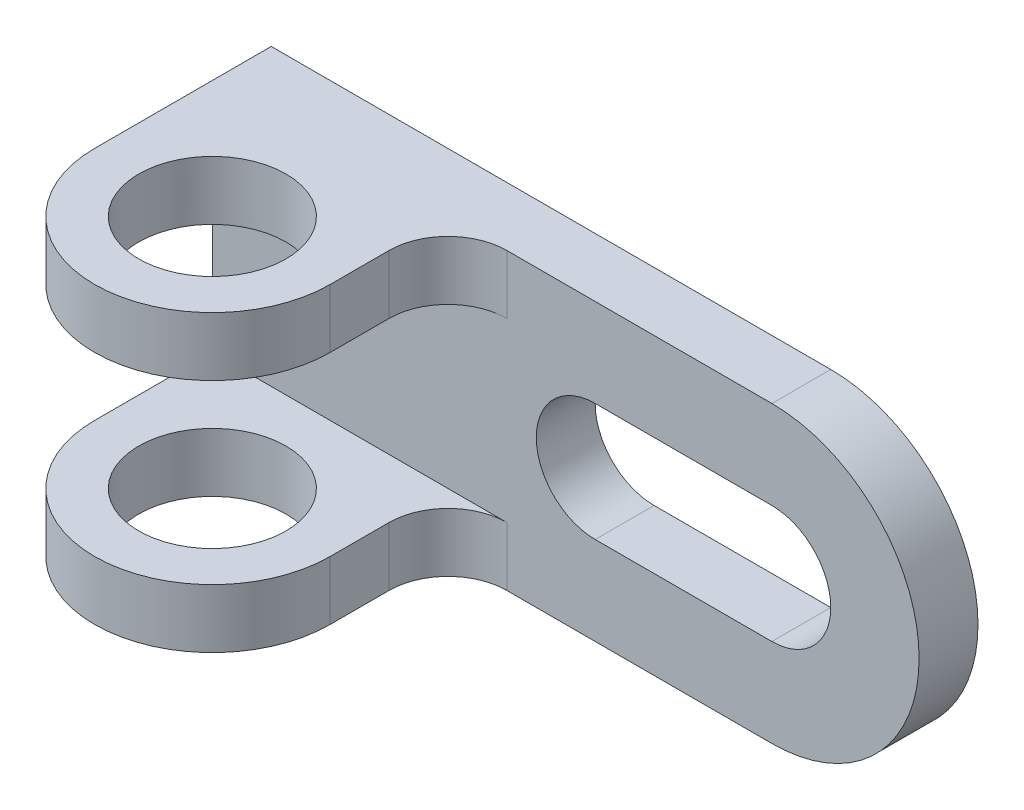
ISO-10303-21;
HEADER;
FILE_DESCRIPTION(('STEP AP214'),'2;1');
FILE_NAME('part.step','',(''),(''),'','','');
FILE_SCHEMA(('AUTOMOTIVE_DESIGN { 1 0 10303 214 1 1 1 1 }'));
ENDSEC;
DATA;
#1=APPLICATION_CONTEXT('core data for automotive mechanical design processes');
#2=APPLICATION_PROTOCOL_DEFINITION('international standard','automotive_design',2000,#1);
#3=PRODUCT_CONTEXT('',#1,'mechanical');
#4=PRODUCT('Part','Part','',(#3));
#5=PRODUCT_RELATED_PRODUCT_CATEGORY('part','',(#4));
#6=PRODUCT_DEFINITION_FORMATION('','',#4);
#7=PRODUCT_DEFINITION_CONTEXT('part definition',#1,'design');
#8=PRODUCT_DEFINITION('design','',#6,#7);
#9=PRODUCT_DEFINITION_SHAPE('','',#8);
#10=(LENGTH_UNIT() NAMED_UNIT(*) SI_UNIT(.MILLI.,.METRE.));
#11=(NAMED_UNIT(*) PLANE_ANGLE_UNIT() SI_UNIT($,.RADIAN.));
#12=(NAMED_UNIT(*) SI_UNIT($,.STERADIAN.) SOLID_ANGLE_UNIT());
#13=UNCERTAINTY_MEASURE_WITH_UNIT(LENGTH_MEASURE(1.E-05),#10,'distance_accuracy_value','');
#14=(GEOMETRIC_REPRESENTATION_CONTEXT(3) GLOBAL_UNCERTAINTY_ASSIGNED_CONTEXT((#13)) GLOBAL_UNIT_ASSIGNED_CONTEXT((#10,
#11,#12)) REPRESENTATION_CONTEXT('',''));
#15=CARTESIAN_POINT('',(0.,0.,0.));
#16=DIRECTION('',(0.,0.,1.));
#17=DIRECTION('',(1.,0.,0.));
#18=AXIS2_PLACEMENT_3D('',#15,#16,#17);
#19=CARTESIAN_POINT('',(95.,0.,10.));
#20=DIRECTION('',(0.,0.,1.));
#21=DIRECTION('',(1.,0.,0.));
#22=AXIS2_PLACEMENT_3D('',#19,#20,#21);
#23=PLANE('',#22);
#24=CARTESIAN_POINT('',(65.,0.,10.));
#25=DIRECTION('',(0.,0.,1.));
#26=DIRECTION('',(1.,0.,0.));
#27=AXIS2_PLACEMENT_3D('',#24,#25,#26);
#28=CIRCLE('',#27,10.);
#29=CARTESIAN_POINT('',(65.,10.,10.));
#30=VERTEX_POINT('',#29);
#31=CARTESIAN_POINT('',(65.,-10.,10.));
#32=VERTEX_POINT('',#31);
#33=EDGE_CURVE('E227',#30,#32,#28,.T.);
#34=ORIENTED_EDGE('',*,*,#33,.F.);
#35=DIRECTION('',(-1.,0.,0.));
#36=VECTOR('',#35,1.);
#37=CARTESIAN_POINT('',(65.,10.,10.));
#38=LINE('',#37,#36);
#39=CARTESIAN_POINT('',(95.,10.,10.));
#40=VERTEX_POINT('',#39);
#41=EDGE_CURVE('E236',#40,#30,#38,.T.);
#42=ORIENTED_EDGE('',*,*,#41,.F.);
#43=CARTESIAN_POINT('',(95.,0.,10.));
#44=DIRECTION('',(0.,0.,1.));
#45=DIRECTION('',(1.,0.,0.));
#46=AXIS2_PLACEMENT_3D('',#43,#44,#45);
#47=CIRCLE('',#46,10.);
#48=CARTESIAN_POINT('',(95.,-10.,10.));
#49=VERTEX_POINT('',#48);
#50=EDGE_CURVE('E252',#49,#40,#47,.T.);
#51=ORIENTED_EDGE('',*,*,#50,.F.);
#52=DIRECTION('',(1.,0.,0.));
#53=VECTOR('',#52,1.);
#54=CARTESIAN_POINT('',(95.,-10.,10.));
#55=LINE('',#54,#53);
#56=EDGE_CURVE('E246',#32,#49,#55,.T.);
#57=ORIENTED_EDGE('',*,*,#56,.F.);
#58=EDGE_LOOP('',(#34,#42,#51,#57));
#59=FACE_BOUND('',#58,.T.);
#60=DIRECTION('',(-1.,0.,0.));
#61=VECTOR('',#60,1.);
#62=CARTESIAN_POINT('',(95.,25.,10.));
#63=LINE('',#62,#61);
#64=CARTESIAN_POINT('',(95.,25.,10.));
#65=VERTEX_POINT('',#64);
#66=CARTESIAN_POINT('',(50.0000000000001,25.,10.));
#67=VERTEX_POINT('',#66);
#68=EDGE_CURVE('E267',#65,#67,#63,.T.);
#69=ORIENTED_EDGE('',*,*,#68,.T.);
#70=DIRECTION('',(0.,1.,0.));
#71=VECTOR('',#70,1.);
#72=CARTESIAN_POINT('',(50.0000000000001,15.,10.));
#73=LINE('',#72,#71);
#74=CARTESIAN_POINT('',(50.0000000000001,15.,10.));
#75=VERTEX_POINT('',#74);
#76=EDGE_CURVE('E62',#75,#67,#73,.T.);
#77=ORIENTED_EDGE('',*,*,#76,.F.);
#78=DIRECTION('',(-1.,0.,0.));
#79=VECTOR('',#78,1.);
#80=CARTESIAN_POINT('',(0.,15.,10.));
#81=LINE('',#80,#79);
#82=CARTESIAN_POINT('',(0.,15.,10.));
#83=VERTEX_POINT('',#82);
#84=EDGE_CURVE('E61',#75,#83,#81,.T.);
#85=ORIENTED_EDGE('',*,*,#84,.T.);
#86=DIRECTION('',(0.,-1.,0.));
#87=VECTOR('',#86,1.);
#88=CARTESIAN_POINT('',(0.,25.,10.));
#89=LINE('',#88,#87);
#90=CARTESIAN_POINT('',(0.,-15.,10.));
#91=VERTEX_POINT('',#90);
#92=EDGE_CURVE('E275',#83,#91,#89,.T.);
#93=ORIENTED_EDGE('',*,*,#92,.T.);
#94=DIRECTION('',(1.,0.,0.));
#95=VECTOR('',#94,1.);
#96=CARTESIAN_POINT('',(0.,-15.,10.));
#97=LINE('',#96,#95);
#98=CARTESIAN_POINT('',(50.0000000000001,-15.,10.));
#99=VERTEX_POINT('',#98);
#100=EDGE_CURVE('E208',#91,#99,#97,.T.);
#101=ORIENTED_EDGE('',*,*,#100,.T.);
#102=DIRECTION('',(0.,-1.,0.));
#103=VECTOR('',#102,1.);
#104=CARTESIAN_POINT('',(50.0000000000001,-15.,10.));
#105=LINE('',#104,#103);
#106=CARTESIAN_POINT('',(50.0000000000001,-25.,10.));
#107=VERTEX_POINT('',#106);
#108=EDGE_CURVE('E229',#99,#107,#105,.T.);
#109=ORIENTED_EDGE('',*,*,#108,.T.);
#110=DIRECTION('',(1.,0.,0.));
#111=VECTOR('',#110,1.);
#112=CARTESIAN_POINT('',(0.,-25.,10.));
#113=LINE('',#112,#111);
#114=CARTESIAN_POINT('',(95.,-25.,10.));
#115=VERTEX_POINT('',#114);
#116=EDGE_CURVE('E273',#107,#115,#113,.T.);
#117=ORIENTED_EDGE('',*,*,#116,.T.);
#118=CARTESIAN_POINT('',(95.,0.,10.));
#119=DIRECTION('',(0.,0.,1.));
#120=DIRECTION('',(1.,0.,0.));
#121=AXIS2_PLACEMENT_3D('',#118,#119,#120);
#122=CIRCLE('',#121,25.);
#123=EDGE_CURVE('E266',#115,#65,#122,.T.);
#124=ORIENTED_EDGE('',*,*,#123,.T.);
#125=EDGE_LOOP('',(#69,#77,#85,#93,#101,#109,#117,#124));
#126=FACE_BOUND('',#125,.T.);
#127=ADVANCED_FACE('F44',(#59,#126),#23,.T.);
#128=CARTESIAN_POINT('',(95.,0.,10.));
#129=DIRECTION('',(0.,0.,-1.));
#130=DIRECTION('',(-1.,0.,0.));
#131=AXIS2_PLACEMENT_3D('',#128,#129,#130);
#132=CYLINDRICAL_SURFACE('',#131,25.);
#133=CARTESIAN_POINT('',(95.,0.,0.));
#134=DIRECTION('',(0.,0.,1.));
#135=DIRECTION('',(1.,0.,0.));
#136=AXIS2_PLACEMENT_3D('',#133,#134,#135);
#137=CIRCLE('',#136,25.);
#138=CARTESIAN_POINT('',(95.,-25.,0.));
#139=VERTEX_POINT('',#138);
#140=CARTESIAN_POINT('',(95.,25.,0.));
#141=VERTEX_POINT('',#140);
#142=EDGE_CURVE('E259',#139,#141,#137,.T.);
#143=ORIENTED_EDGE('',*,*,#142,.T.);
#144=DIRECTION('',(0.,0.,-1.));
#145=VECTOR('',#144,1.);
#146=CARTESIAN_POINT('',(95.,25.,10.));
#147=LINE('',#146,#145);
#148=EDGE_CURVE('E11',#65,#141,#147,.T.);
#149=ORIENTED_EDGE('',*,*,#148,.F.);
#150=ORIENTED_EDGE('',*,*,#123,.F.);
#151=DIRECTION('',(0.,0.,-1.));
#152=VECTOR('',#151,1.);
#153=CARTESIAN_POINT('',(95.,-25.,10.));
#154=LINE('',#153,#152);
#155=EDGE_CURVE('E277',#115,#139,#154,.T.);
#156=ORIENTED_EDGE('',*,*,#155,.T.);
#157=EDGE_LOOP('',(#143,#149,#150,#156));
#158=FACE_BOUND('',#157,.T.);
#159=ADVANCED_FACE('F50',(#158),#132,.T.);
#160=CARTESIAN_POINT('',(95.,25.,10.));
#161=DIRECTION('',(0.,-1.,0.));
#162=DIRECTION('',(0.,0.,-1.));
#163=AXIS2_PLACEMENT_3D('',#160,#161,#162);
#164=PLANE('',#163);
#165=CARTESIAN_POINT('',(20.,25.,30.));
#166=DIRECTION('',(0.,-1.,0.));
#167=DIRECTION('',(0.,0.,-1.));
#168=AXIS2_PLACEMENT_3D('',#165,#166,#167);
#169=CIRCLE('',#168,12.5);
#170=CARTESIAN_POINT('',(20.,25.,17.5));
#171=VERTEX_POINT('',#170);
#172=EDGE_CURVE('E356',#171,#171,#169,.T.);
#173=ORIENTED_EDGE('',*,*,#172,.T.);
#174=EDGE_LOOP('',(#173));
#175=FACE_BOUND('',#174,.T.);
#176=DIRECTION('',(-1.,0.,0.));
#177=VECTOR('',#176,1.);
#178=CARTESIAN_POINT('',(95.,25.,0.));
#179=LINE('',#178,#177);
#180=CARTESIAN_POINT('',(0.,25.,0.));
#181=VERTEX_POINT('',#180);
#182=EDGE_CURVE('E276',#141,#181,#179,.T.);
#183=ORIENTED_EDGE('',*,*,#182,.T.);
#184=DIRECTION('',(0.,0.,-1.));
#185=VECTOR('',#184,1.);
#186=CARTESIAN_POINT('',(0.,25.,10.));
#187=LINE('',#186,#185);
#188=CARTESIAN_POINT('',(0.,25.,30.));
#189=VERTEX_POINT('',#188);
#190=EDGE_CURVE('E53',#189,#181,#187,.T.);
#191=ORIENTED_EDGE('',*,*,#190,.F.);
#192=CARTESIAN_POINT('',(20.,25.,30.));
#193=DIRECTION('',(0.,1.,0.));
#194=DIRECTION('',(0.,0.,1.));
#195=AXIS2_PLACEMENT_3D('',#192,#193,#194);
#196=CIRCLE('',#195,20.);
#197=CARTESIAN_POINT('',(40.,25.,30.));
#198=VERTEX_POINT('',#197);
#199=EDGE_CURVE('E191',#189,#198,#196,.T.);
#200=ORIENTED_EDGE('',*,*,#199,.T.);
#201=DIRECTION('',(0.,0.,-1.));
#202=VECTOR('',#201,1.);
#203=CARTESIAN_POINT('',(40.,25.,30.));
#204=LINE('',#203,#202);
#205=CARTESIAN_POINT('',(40.,25.,20.0000000000001));
#206=VERTEX_POINT('',#205);
#207=EDGE_CURVE('E165',#198,#206,#204,.T.);
#208=ORIENTED_EDGE('',*,*,#207,.T.);
#209=CARTESIAN_POINT('',(50.,25.,20.));
#210=DIRECTION('',(0.,-1.,0.));
#211=DIRECTION('',(0.,0.,1.));
#212=AXIS2_PLACEMENT_3D('',#209,#210,#211);
#213=CIRCLE('',#212,10.);
#214=EDGE_CURVE('E181',#206,#67,#213,.T.);
#215=ORIENTED_EDGE('',*,*,#214,.T.);
#216=ORIENTED_EDGE('',*,*,#68,.F.);
#217=ORIENTED_EDGE('',*,*,#148,.T.);
#218=EDGE_LOOP('',(#183,#191,#200,#208,#215,#216,#217));
#219=FACE_BOUND('',#218,.T.);
#220=ADVANCED_FACE('F339',(#175,#219),#164,.F.);
#221=CARTESIAN_POINT('',(0.,25.,10.));
#222=DIRECTION('',(1.,0.,0.));
#223=DIRECTION('',(0.,0.,-1.));
#224=AXIS2_PLACEMENT_3D('',#221,#222,#223);
#225=PLANE('',#224);
#226=DIRECTION('',(0.,-1.,0.));
#227=VECTOR('',#226,1.);
#228=CARTESIAN_POINT('',(0.,25.,0.));
#229=LINE('',#228,#227);
#230=CARTESIAN_POINT('',(0.,-25.,0.));
#231=VERTEX_POINT('',#230);
#232=EDGE_CURVE('E282',#181,#231,#229,.T.);
#233=ORIENTED_EDGE('',*,*,#232,.T.);
#234=DIRECTION('',(0.,0.,-1.));
#235=VECTOR('',#234,1.);
#236=CARTESIAN_POINT('',(0.,-25.,10.));
#237=LINE('',#236,#235);
#238=CARTESIAN_POINT('',(0.,-25.,30.));
#239=VERTEX_POINT('',#238);
#240=EDGE_CURVE('E287',#239,#231,#237,.T.);
#241=ORIENTED_EDGE('',*,*,#240,.F.);
#242=DIRECTION('',(0.,-1.,0.));
#243=VECTOR('',#242,1.);
#244=CARTESIAN_POINT('',(0.,-15.,30.));
#245=LINE('',#244,#243);
#246=CARTESIAN_POINT('',(0.,-15.,30.));
#247=VERTEX_POINT('',#246);
#248=EDGE_CURVE('E216',#247,#239,#245,.T.);
#249=ORIENTED_EDGE('',*,*,#248,.F.);
#250=DIRECTION('',(0.,0.,-1.));
#251=VECTOR('',#250,1.);
#252=CARTESIAN_POINT('',(0.,-15.,10.));
#253=LINE('',#252,#251);
#254=EDGE_CURVE('E204',#247,#91,#253,.T.);
#255=ORIENTED_EDGE('',*,*,#254,.T.);
#256=ORIENTED_EDGE('',*,*,#92,.F.);
#257=DIRECTION('',(0.,0.,1.));
#258=VECTOR('',#257,1.);
#259=CARTESIAN_POINT('',(0.,15.,30.));
#260=LINE('',#259,#258);
#261=CARTESIAN_POINT('',(0.,15.,30.));
#262=VERTEX_POINT('',#261);
#263=EDGE_CURVE('E169',#83,#262,#260,.T.);
#264=ORIENTED_EDGE('',*,*,#263,.T.);
#265=DIRECTION('',(0.,1.,0.));
#266=VECTOR('',#265,1.);
#267=CARTESIAN_POINT('',(0.,15.,30.));
#268=LINE('',#267,#266);
#269=EDGE_CURVE('E185',#262,#189,#268,.T.);
#270=ORIENTED_EDGE('',*,*,#269,.T.);
#271=ORIENTED_EDGE('',*,*,#190,.T.);
#272=EDGE_LOOP('',(#233,#241,#249,#255,#256,#264,#270,#271));
#273=FACE_BOUND('',#272,.T.);
#274=ADVANCED_FACE('F295',(#273),#225,.F.);
#275=CARTESIAN_POINT('',(0.,-25.,10.));
#276=DIRECTION('',(0.,1.,0.));
#277=DIRECTION('',(0.,0.,1.));
#278=AXIS2_PLACEMENT_3D('',#275,#276,#277);
#279=PLANE('',#278);
#280=CARTESIAN_POINT('',(20.,-25.,30.));
#281=DIRECTION('',(0.,-1.,0.));
#282=DIRECTION('',(0.,0.,-1.));
#283=AXIS2_PLACEMENT_3D('',#280,#281,#282);
#284=CIRCLE('',#283,12.5);
#285=CARTESIAN_POINT('',(20.,-25.,17.5));
#286=VERTEX_POINT('',#285);
#287=EDGE_CURVE('E387',#286,#286,#284,.T.);
#288=ORIENTED_EDGE('',*,*,#287,.F.);
#289=EDGE_LOOP('',(#288));
#290=FACE_BOUND('',#289,.T.);
#291=DIRECTION('',(1.,0.,0.));
#292=VECTOR('',#291,1.);
#293=CARTESIAN_POINT('',(0.,-25.,0.));
#294=LINE('',#293,#292);
#295=EDGE_CURVE('E269',#231,#139,#294,.T.);
#296=ORIENTED_EDGE('',*,*,#295,.T.);
#297=ORIENTED_EDGE('',*,*,#155,.F.);
#298=ORIENTED_EDGE('',*,*,#116,.F.);
#299=CARTESIAN_POINT('',(50.,-25.,20.));
#300=DIRECTION('',(0.,1.,0.));
#301=DIRECTION('',(0.,0.,1.));
#302=AXIS2_PLACEMENT_3D('',#299,#300,#301);
#303=CIRCLE('',#302,10.);
#304=CARTESIAN_POINT('',(40.,-25.,20.0000000000001));
#305=VERTEX_POINT('',#304);
#306=EDGE_CURVE('E218',#107,#305,#303,.T.);
#307=ORIENTED_EDGE('',*,*,#306,.T.);
#308=DIRECTION('',(0.,0.,1.));
#309=VECTOR('',#308,1.);
#310=CARTESIAN_POINT('',(40.,-25.,30.));
#311=LINE('',#310,#309);
#312=CARTESIAN_POINT('',(40.,-25.,30.));
#313=VERTEX_POINT('',#312);
#314=EDGE_CURVE('E202',#305,#313,#311,.T.);
#315=ORIENTED_EDGE('',*,*,#314,.T.);
#316=CARTESIAN_POINT('',(20.,-25.,30.));
#317=DIRECTION('',(0.,-1.,0.));
#318=DIRECTION('',(0.,0.,-1.));
#319=AXIS2_PLACEMENT_3D('',#316,#317,#318);
#320=CIRCLE('',#319,20.);
#321=EDGE_CURVE('E196',#313,#239,#320,.T.);
#322=ORIENTED_EDGE('',*,*,#321,.T.);
#323=ORIENTED_EDGE('',*,*,#240,.T.);
#324=EDGE_LOOP('',(#296,#297,#298,#307,#315,#322,#323));
#325=FACE_BOUND('',#324,.T.);
#326=ADVANCED_FACE('F296',(#290,#325),#279,.F.);
#327=CARTESIAN_POINT('',(95.,0.,0.));
#328=DIRECTION('',(0.,0.,1.));
#329=DIRECTION('',(1.,0.,0.));
#330=AXIS2_PLACEMENT_3D('',#327,#328,#329);
#331=PLANE('',#330);
#332=DIRECTION('',(-1.,0.,0.));
#333=VECTOR('',#332,1.);
#334=CARTESIAN_POINT('',(65.,10.,0.));
#335=LINE('',#334,#333);
#336=CARTESIAN_POINT('',(95.,10.,0.));
#337=VERTEX_POINT('',#336);
#338=CARTESIAN_POINT('',(65.,10.,0.));
#339=VERTEX_POINT('',#338);
#340=EDGE_CURVE('E244',#337,#339,#335,.T.);
#341=ORIENTED_EDGE('',*,*,#340,.T.);
#342=CARTESIAN_POINT('',(65.,0.,0.));
#343=DIRECTION('',(0.,0.,1.));
#344=DIRECTION('',(1.,0.,0.));
#345=AXIS2_PLACEMENT_3D('',#342,#343,#344);
#346=CIRCLE('',#345,10.);
#347=CARTESIAN_POINT('',(65.,-10.,0.));
#348=VERTEX_POINT('',#347);
#349=EDGE_CURVE('E231',#339,#348,#346,.T.);
#350=ORIENTED_EDGE('',*,*,#349,.T.);
#351=DIRECTION('',(1.,0.,0.));
#352=VECTOR('',#351,1.);
#353=CARTESIAN_POINT('',(95.,-10.,0.));
#354=LINE('',#353,#352);
#355=CARTESIAN_POINT('',(95.,-10.,0.));
#356=VERTEX_POINT('',#355);
#357=EDGE_CURVE('E240',#348,#356,#354,.T.);
#358=ORIENTED_EDGE('',*,*,#357,.T.);
#359=CARTESIAN_POINT('',(95.,0.,0.));
#360=DIRECTION('',(0.,0.,1.));
#361=DIRECTION('',(1.,0.,0.));
#362=AXIS2_PLACEMENT_3D('',#359,#360,#361);
#363=CIRCLE('',#362,10.);
#364=EDGE_CURVE('E242',#356,#337,#363,.T.);
#365=ORIENTED_EDGE('',*,*,#364,.T.);
#366=EDGE_LOOP('',(#341,#350,#358,#365));
#367=FACE_BOUND('',#366,.T.);
#368=ORIENTED_EDGE('',*,*,#142,.F.);
#369=ORIENTED_EDGE('',*,*,#295,.F.);
#370=ORIENTED_EDGE('',*,*,#232,.F.);
#371=ORIENTED_EDGE('',*,*,#182,.F.);
#372=EDGE_LOOP('',(#368,#369,#370,#371));
#373=FACE_BOUND('',#372,.T.);
#374=ADVANCED_FACE('F300',(#367,#373),#331,.F.);
#375=CARTESIAN_POINT('',(65.,0.,0.));
#376=DIRECTION('',(0.,0.,1.));
#377=DIRECTION('',(1.,0.,0.));
#378=AXIS2_PLACEMENT_3D('',#375,#376,#377);
#379=CYLINDRICAL_SURFACE('',#378,10.);
#380=ORIENTED_EDGE('',*,*,#33,.T.);
#381=DIRECTION('',(0.,0.,1.));
#382=VECTOR('',#381,1.);
#383=CARTESIAN_POINT('',(65.,-10.,0.));
#384=LINE('',#383,#382);
#385=EDGE_CURVE('E250',#348,#32,#384,.T.);
#386=ORIENTED_EDGE('',*,*,#385,.F.);
#387=ORIENTED_EDGE('',*,*,#349,.F.);
#388=DIRECTION('',(0.,0.,1.));
#389=VECTOR('',#388,1.);
#390=CARTESIAN_POINT('',(65.,10.,0.));
#391=LINE('',#390,#389);
#392=EDGE_CURVE('E260',#339,#30,#391,.T.);
#393=ORIENTED_EDGE('',*,*,#392,.T.);
#394=EDGE_LOOP('',(#380,#386,#387,#393));
#395=FACE_BOUND('',#394,.T.);
#396=ADVANCED_FACE('F344',(#395),#379,.F.);
#397=CARTESIAN_POINT('',(65.,10.,0.));
#398=DIRECTION('',(0.,1.,0.));
#399=DIRECTION('',(0.,0.,1.));
#400=AXIS2_PLACEMENT_3D('',#397,#398,#399);
#401=PLANE('',#400);
#402=ORIENTED_EDGE('',*,*,#41,.T.);
#403=ORIENTED_EDGE('',*,*,#392,.F.);
#404=ORIENTED_EDGE('',*,*,#340,.F.);
#405=DIRECTION('',(0.,0.,1.));
#406=VECTOR('',#405,1.);
#407=CARTESIAN_POINT('',(95.,10.,0.));
#408=LINE('',#407,#406);
#409=EDGE_CURVE('E257',#337,#40,#408,.T.);
#410=ORIENTED_EDGE('',*,*,#409,.T.);
#411=EDGE_LOOP('',(#402,#403,#404,#410));
#412=FACE_BOUND('',#411,.T.);
#413=ADVANCED_FACE('F454',(#412),#401,.F.);
#414=CARTESIAN_POINT('',(95.,0.,0.));
#415=DIRECTION('',(0.,0.,1.));
#416=DIRECTION('',(1.,0.,0.));
#417=AXIS2_PLACEMENT_3D('',#414,#415,#416);
#418=CYLINDRICAL_SURFACE('',#417,10.);
#419=ORIENTED_EDGE('',*,*,#50,.T.);
#420=ORIENTED_EDGE('',*,*,#409,.F.);
#421=ORIENTED_EDGE('',*,*,#364,.F.);
#422=DIRECTION('',(0.,0.,1.));
#423=VECTOR('',#422,1.);
#424=CARTESIAN_POINT('',(95.,-10.,0.));
#425=LINE('',#424,#423);
#426=EDGE_CURVE('E265',#356,#49,#425,.T.);
#427=ORIENTED_EDGE('',*,*,#426,.T.);
#428=EDGE_LOOP('',(#419,#420,#421,#427));
#429=FACE_BOUND('',#428,.T.);
#430=ADVANCED_FACE('F441',(#429),#418,.F.);
#431=CARTESIAN_POINT('',(95.,-10.,0.));
#432=DIRECTION('',(0.,-1.,0.));
#433=DIRECTION('',(0.,0.,-1.));
#434=AXIS2_PLACEMENT_3D('',#431,#432,#433);
#435=PLANE('',#434);
#436=ORIENTED_EDGE('',*,*,#56,.T.);
#437=ORIENTED_EDGE('',*,*,#426,.F.);
#438=ORIENTED_EDGE('',*,*,#357,.F.);
#439=ORIENTED_EDGE('',*,*,#385,.T.);
#440=EDGE_LOOP('',(#436,#437,#438,#439));
#441=FACE_BOUND('',#440,.T.);
#442=ADVANCED_FACE('F436',(#441),#435,.F.);
#443=CARTESIAN_POINT('',(20.,-15.,30.));
#444=DIRECTION('',(0.,-1.,0.));
#445=DIRECTION('',(0.,0.,-1.));
#446=AXIS2_PLACEMENT_3D('',#443,#444,#445);
#447=CYLINDRICAL_SURFACE('',#446,20.);
#448=ORIENTED_EDGE('',*,*,#321,.F.);
#449=DIRECTION('',(0.,-1.,0.));
#450=VECTOR('',#449,1.);
#451=CARTESIAN_POINT('',(40.,-15.,30.));
#452=LINE('',#451,#450);
#453=CARTESIAN_POINT('',(40.,-15.,30.));
#454=VERTEX_POINT('',#453);
#455=EDGE_CURVE('E221',#454,#313,#452,.T.);
#456=ORIENTED_EDGE('',*,*,#455,.F.);
#457=CARTESIAN_POINT('',(20.,-15.,30.));
#458=DIRECTION('',(0.,-1.,0.));
#459=DIRECTION('',(0.,0.,-1.));
#460=AXIS2_PLACEMENT_3D('',#457,#458,#459);
#461=CIRCLE('',#460,20.);
#462=EDGE_CURVE('E203',#454,#247,#461,.T.);
#463=ORIENTED_EDGE('',*,*,#462,.T.);
#464=ORIENTED_EDGE('',*,*,#248,.T.);
#465=EDGE_LOOP('',(#448,#456,#463,#464));
#466=FACE_BOUND('',#465,.T.);
#467=ADVANCED_FACE('F314',(#466),#447,.T.);
#468=CARTESIAN_POINT('',(40.,-15.,30.));
#469=DIRECTION('',(1.,0.,0.));
#470=DIRECTION('',(0.,0.,-1.));
#471=AXIS2_PLACEMENT_3D('',#468,#469,#470);
#472=PLANE('',#471);
#473=ORIENTED_EDGE('',*,*,#314,.F.);
#474=DIRECTION('',(0.,-1.,0.));
#475=VECTOR('',#474,1.);
#476=CARTESIAN_POINT('',(40.,-15.,20.0000000000001));
#477=LINE('',#476,#475);
#478=CARTESIAN_POINT('',(40.,-15.,20.0000000000001));
#479=VERTEX_POINT('',#478);
#480=EDGE_CURVE('E230',#479,#305,#477,.T.);
#481=ORIENTED_EDGE('',*,*,#480,.F.);
#482=DIRECTION('',(0.,0.,1.));
#483=VECTOR('',#482,1.);
#484=CARTESIAN_POINT('',(40.,-15.,30.));
#485=LINE('',#484,#483);
#486=EDGE_CURVE('E213',#479,#454,#485,.T.);
#487=ORIENTED_EDGE('',*,*,#486,.T.);
#488=ORIENTED_EDGE('',*,*,#455,.T.);
#489=EDGE_LOOP('',(#473,#481,#487,#488));
#490=FACE_BOUND('',#489,.T.);
#491=ADVANCED_FACE('F310',(#490),#472,.T.);
#492=CARTESIAN_POINT('',(50.,-15.,20.));
#493=DIRECTION('',(0.,-1.,0.));
#494=DIRECTION('',(0.,0.,-1.));
#495=AXIS2_PLACEMENT_3D('',#492,#493,#494);
#496=CYLINDRICAL_SURFACE('',#495,10.);
#497=ORIENTED_EDGE('',*,*,#306,.F.);
#498=ORIENTED_EDGE('',*,*,#108,.F.);
#499=CARTESIAN_POINT('',(50.,-15.,20.));
#500=DIRECTION('',(0.,1.,0.));
#501=DIRECTION('',(0.,0.,1.));
#502=AXIS2_PLACEMENT_3D('',#499,#500,#501);
#503=CIRCLE('',#502,10.);
#504=EDGE_CURVE('E209',#99,#479,#503,.T.);
#505=ORIENTED_EDGE('',*,*,#504,.T.);
#506=ORIENTED_EDGE('',*,*,#480,.T.);
#507=EDGE_LOOP('',(#497,#498,#505,#506));
#508=FACE_BOUND('',#507,.T.);
#509=ADVANCED_FACE('F319',(#508),#496,.F.);
#510=CARTESIAN_POINT('',(20.,-15.,30.));
#511=DIRECTION('',(0.,-1.,0.));
#512=DIRECTION('',(0.,0.,-1.));
#513=AXIS2_PLACEMENT_3D('',#510,#511,#512);
#514=PLANE('',#513);
#515=CARTESIAN_POINT('',(20.,-15.,30.));
#516=DIRECTION('',(0.,-1.,0.));
#517=DIRECTION('',(0.,0.,-1.));
#518=AXIS2_PLACEMENT_3D('',#515,#516,#517);
#519=CIRCLE('',#518,12.5);
#520=CARTESIAN_POINT('',(20.,-15.,17.5));
#521=VERTEX_POINT('',#520);
#522=EDGE_CURVE('E188',#521,#521,#519,.T.);
#523=ORIENTED_EDGE('',*,*,#522,.T.);
#524=EDGE_LOOP('',(#523));
#525=FACE_BOUND('',#524,.T.);
#526=ORIENTED_EDGE('',*,*,#462,.F.);
#527=ORIENTED_EDGE('',*,*,#486,.F.);
#528=ORIENTED_EDGE('',*,*,#504,.F.);
#529=ORIENTED_EDGE('',*,*,#100,.F.);
#530=ORIENTED_EDGE('',*,*,#254,.F.);
#531=EDGE_LOOP('',(#526,#527,#528,#529,#530));
#532=FACE_BOUND('',#531,.T.);
#533=ADVANCED_FACE('F318',(#525,#532),#514,.F.);
#534=CARTESIAN_POINT('',(20.,15.,30.));
#535=DIRECTION('',(0.,1.,0.));
#536=DIRECTION('',(0.,0.,1.));
#537=AXIS2_PLACEMENT_3D('',#534,#535,#536);
#538=CYLINDRICAL_SURFACE('',#537,20.);
#539=ORIENTED_EDGE('',*,*,#199,.F.);
#540=ORIENTED_EDGE('',*,*,#269,.F.);
#541=CARTESIAN_POINT('',(20.,15.,30.));
#542=DIRECTION('',(0.,1.,0.));
#543=DIRECTION('',(0.,0.,1.));
#544=AXIS2_PLACEMENT_3D('',#541,#542,#543);
#545=CIRCLE('',#544,20.);
#546=CARTESIAN_POINT('',(40.,15.,30.));
#547=VERTEX_POINT('',#546);
#548=EDGE_CURVE('E171',#262,#547,#545,.T.);
#549=ORIENTED_EDGE('',*,*,#548,.T.);
#550=DIRECTION('',(0.,1.,0.));
#551=VECTOR('',#550,1.);
#552=CARTESIAN_POINT('',(40.,15.,30.));
#553=LINE('',#552,#551);
#554=EDGE_CURVE('E160',#547,#198,#553,.T.);
#555=ORIENTED_EDGE('',*,*,#554,.T.);
#556=EDGE_LOOP('',(#539,#540,#549,#555));
#557=FACE_BOUND('',#556,.T.);
#558=ADVANCED_FACE('F178',(#557),#538,.T.);
#559=CARTESIAN_POINT('',(50.,15.,20.));
#560=DIRECTION('',(0.,1.,0.));
#561=DIRECTION('',(0.,0.,1.));
#562=AXIS2_PLACEMENT_3D('',#559,#560,#561);
#563=CYLINDRICAL_SURFACE('',#562,10.);
#564=ORIENTED_EDGE('',*,*,#214,.F.);
#565=DIRECTION('',(0.,1.,0.));
#566=VECTOR('',#565,1.);
#567=CARTESIAN_POINT('',(40.,15.,20.0000000000001));
#568=LINE('',#567,#566);
#569=CARTESIAN_POINT('',(40.,15.,20.0000000000001));
#570=VERTEX_POINT('',#569);
#571=EDGE_CURVE('E170',#570,#206,#568,.T.);
#572=ORIENTED_EDGE('',*,*,#571,.F.);
#573=CARTESIAN_POINT('',(50.,15.,20.));
#574=DIRECTION('',(0.,-1.,0.));
#575=DIRECTION('',(0.,0.,1.));
#576=AXIS2_PLACEMENT_3D('',#573,#574,#575);
#577=CIRCLE('',#576,10.);
#578=EDGE_CURVE('E179',#570,#75,#577,.T.);
#579=ORIENTED_EDGE('',*,*,#578,.T.);
#580=ORIENTED_EDGE('',*,*,#76,.T.);
#581=EDGE_LOOP('',(#564,#572,#579,#580));
#582=FACE_BOUND('',#581,.T.);
#583=ADVANCED_FACE('F362',(#582),#563,.F.);
#584=CARTESIAN_POINT('',(40.,15.,30.));
#585=DIRECTION('',(1.,0.,0.));
#586=DIRECTION('',(0.,0.,-1.));
#587=AXIS2_PLACEMENT_3D('',#584,#585,#586);
#588=PLANE('',#587);
#589=ORIENTED_EDGE('',*,*,#207,.F.);
#590=ORIENTED_EDGE('',*,*,#554,.F.);
#591=DIRECTION('',(0.,0.,-1.));
#592=VECTOR('',#591,1.);
#593=CARTESIAN_POINT('',(40.,15.,30.));
#594=LINE('',#593,#592);
#595=EDGE_CURVE('E159',#547,#570,#594,.T.);
#596=ORIENTED_EDGE('',*,*,#595,.T.);
#597=ORIENTED_EDGE('',*,*,#571,.T.);
#598=EDGE_LOOP('',(#589,#590,#596,#597));
#599=FACE_BOUND('',#598,.T.);
#600=ADVANCED_FACE('F157',(#599),#588,.T.);
#601=CARTESIAN_POINT('',(20.,15.,30.));
#602=DIRECTION('',(0.,1.,0.));
#603=DIRECTION('',(0.,0.,1.));
#604=AXIS2_PLACEMENT_3D('',#601,#602,#603);
#605=PLANE('',#604);
#606=CARTESIAN_POINT('',(20.,15.,30.));
#607=DIRECTION('',(0.,1.,0.));
#608=DIRECTION('',(0.,0.,1.));
#609=AXIS2_PLACEMENT_3D('',#606,#607,#608);
#610=CIRCLE('',#609,12.5);
#611=CARTESIAN_POINT('',(20.,15.,42.5));
#612=VERTEX_POINT('',#611);
#613=EDGE_CURVE('E47',#612,#612,#610,.T.);
#614=ORIENTED_EDGE('',*,*,#613,.T.);
#615=EDGE_LOOP('',(#614));
#616=FACE_BOUND('',#615,.T.);
#617=ORIENTED_EDGE('',*,*,#548,.F.);
#618=ORIENTED_EDGE('',*,*,#263,.F.);
#619=ORIENTED_EDGE('',*,*,#84,.F.);
#620=ORIENTED_EDGE('',*,*,#578,.F.);
#621=ORIENTED_EDGE('',*,*,#595,.F.);
#622=EDGE_LOOP('',(#617,#618,#619,#620,#621));
#623=FACE_BOUND('',#622,.T.);
#624=ADVANCED_FACE('F173',(#616,#623),#605,.F.);
#625=CARTESIAN_POINT('',(20.,25.,30.));
#626=DIRECTION('',(0.,-1.,0.));
#627=DIRECTION('',(0.,0.,-1.));
#628=AXIS2_PLACEMENT_3D('',#625,#626,#627);
#629=CYLINDRICAL_SURFACE('',#628,12.5);
#630=ORIENTED_EDGE('',*,*,#172,.F.);
#631=EDGE_LOOP('',(#630));
#632=FACE_BOUND('',#631,.T.);
#633=ORIENTED_EDGE('',*,*,#613,.F.);
#634=EDGE_LOOP('',(#633));
#635=FACE_BOUND('',#634,.T.);
#636=ADVANCED_FACE('F372',(#632,#635),#629,.F.);
#637=ORIENTED_EDGE('',*,*,#287,.T.);
#638=EDGE_LOOP('',(#637));
#639=FACE_BOUND('',#638,.T.);
#640=ORIENTED_EDGE('',*,*,#522,.F.);
#641=EDGE_LOOP('',(#640));
#642=FACE_BOUND('',#641,.T.);
#643=ADVANCED_FACE('F376',(#639,#642),#629,.F.);
#644=CLOSED_SHELL('',(#127,#159,#220,#274,#326,#374,#396,#413,#430,#442,#467,#491,#509,#533,
#558,#583,#600,#624,#636,#643));
#645=MANIFOLD_SOLID_BREP('B2',#644);
#646=ADVANCED_BREP_SHAPE_REPRESENTATION('',(#18,#645),#14);
#647=SHAPE_DEFINITION_REPRESENTATION(#9,#646);
ENDSEC;
END-ISO-10303-21;
